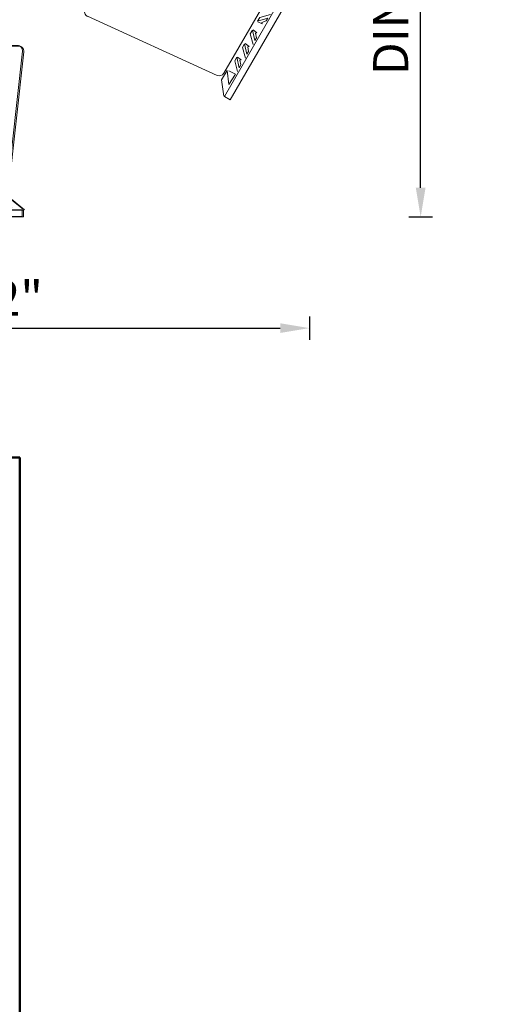
# Model space of a CAD drawing. Units: inches. Extents: x 1961 to 3038, y 800 to 1438.
# Tile 7 of 13: x 2803 to 2845, y 1012 to 1096. Entities that reach past the tile are written whole.
import ezdxf

# ---------------------------------------------------------------- set-up
doc = ezdxf.new("R2010")
doc.units = ezdxf.units.IN
for name, color, linetype, lineweight in [('A-ANNO-DIMS', 2, 'Continuous', 18), ('A-FURN', 8, 'Continuous', 18), ('A-WALL', 7, 'Continuous', 50)]:
    doc.layers.add(name, color=color, linetype=linetype, lineweight=lineweight)
doc.styles.get("Standard").update_dxf_attribs({"font": 'arial.ttf'})
doc.dimstyles.new('ISO-25', dxfattribs={"dimtxt": 3, "dimasz": 2.5, "dimexe": 1, "dimexo": 1, "dimtad": 1, "dimdec": 4, "dimlunit": 4, "dimtxsty": 'Standard', "dimcen": 2.5, "dimadec": 0, "dimazin": 0, "dimtfac": 1, "dimtdec": 4, "dimtmove": 0, "dimatfit": 3, "dimfxl": 1, "dimfxlon": 1, "dimarcsym": 0})

# ---------------------------------------------------------------- blocks, each defined once
blk = doc.blocks.new('A$C1C317F9A')
for p, q in [((0.8788, 2.2685), (0.8788, 2.2478)), ((1.3449, 2.2685), (0.8788, 2.2685)), ((1.3449, 2.2478), (1.3449, 2.2685)), ((0.8756, 2.2462), (0.9155, 2.2143)), ((0.8788, 2.2478), (1.3449, 2.2478)), ((0.9139, 2.2414), (0.9522, 2.243)), ((0.949, 2.2159), (0.9139, 2.2414)), ((0.9522, 2.243), (0.9506, 2.2206)), ((0.9618, 2.2446), (0.9857, 2.2206)), ((0.9745, 2.243), (0.9841, 2.243)), ((0.9985, 2.2206), (0.9745, 2.243)), ((0.9841, 2.243), (0.9953, 2.2334)), ((0.9953, 2.2334), (0.9985, 2.2366)), ((0.9985, 2.2366), (1.0001, 2.2222)), ((1.0097, 2.2446), (1.0336, 2.2206)), ((1.0224, 2.243), (1.032, 2.243)), ((1.0464, 2.2206), (1.0224, 2.243)), ((1.032, 2.243), (1.0432, 2.2334)), ((1.0432, 2.2334), (1.0464, 2.2366)), ((1.0464, 2.2366), (1.048, 2.2222)), ((1.0576, 2.2446), (1.0815, 2.2206)), ((1.0703, 2.243), (1.0799, 2.243)), ((1.0943, 2.2206), (1.0703, 2.243)), ((1.0799, 2.243), (1.0911, 2.2334)), ((1.0911, 2.2334), (1.0943, 2.2366)), ((1.0943, 2.2366), (1.0959, 2.2222)), ((1.1262, 2.2366), (1.1246, 2.2222)), ((1.1262, 2.2206), (1.1502, 2.243)), ((1.1294, 2.2334), (1.1262, 2.2366)), ((1.1406, 2.243), (1.1294, 2.2334)), ((1.1629, 2.2446), (1.139, 2.2206)), ((1.1502, 2.243), (1.1406, 2.243)), ((1.1741, 2.2366), (1.1725, 2.2222)), ((1.1741, 2.2206), (1.1981, 2.243)), ((1.1773, 2.2334), (1.1741, 2.2366)), ((1.1885, 2.243), (1.1773, 2.2334)), ((1.2108, 2.2446), (1.1869, 2.2206)), ((1.1981, 2.243), (1.1885, 2.243)), ((1.222, 2.2366), (1.2204, 2.2222)), ((1.222, 2.2206), (1.246, 2.243)), ((1.2252, 2.2334), (1.222, 2.2366)), ((1.2364, 2.243), (1.2252, 2.2334)), ((1.2587, 2.2446), (1.2348, 2.2206)), ((1.246, 2.243), (1.2364, 2.243)), ((1.2683, 2.243), (1.2699, 2.2206)), ((1.3066, 2.2414), (1.2683, 2.243)), ((1.2715, 2.2159), (1.3066, 2.2414)), ((1.3449, 2.2462), (1.305, 2.2143)), ((0.9155, 2.2143), (0.949, 2.2159)), ((0.941, 2.2111), (1.2841, 2.2111)), ((0.9857, 2.2206), (0.9985, 2.2206)), ((1.0336, 2.2206), (1.0464, 2.2206)), ((1.0815, 2.2206), (1.0943, 2.2206)), ((1.139, 2.2206), (1.1262, 2.2206)), ((1.1869, 2.2206), (1.1741, 2.2206)), ((1.2348, 2.2206), (1.222, 2.2206)), ((1.305, 2.2143), (1.2715, 2.2159)), ((0.8775, 1.7628), (0.9251, 2.1968)), ((1.3, 2.1966), (1.3417, 1.7626)), ((0.2422, 1.9115), (0.0091, 1.5078)), ((0.0271, 1.4974), (0.2602, 1.9011)), ((0.2602, 1.9011), (0.2422, 1.9115)), ((0.2615, 1.9003), (0.2692, 1.8498)), ((1.9514, 1.8873), (1.9438, 1.8368)), ((1.9724, 1.8957), (1.9544, 1.8854)), ((1.9544, 1.8854), (2.1875, 1.4816)), ((2.2055, 1.492), (1.9724, 1.8957)), ((0.2465, 1.8648), (0.226, 1.8324)), ((0.2511, 1.8216), (0.2465, 1.8648)), ((0.2692, 1.8498), (0.2511, 1.8216)), ((1.9619, 1.8086), (1.9665, 1.8518)), ((1.9665, 1.8518), (1.987, 1.8194)), ((0.09, 1.5329), (0.2615, 1.8301)), ((0.2148, 1.813), (0.21, 1.8047)), ((0.2222, 1.7811), (0.2148, 1.813)), ((0.2198, 1.8249), (0.2286, 1.7922)), ((0.226, 1.8324), (0.2461, 1.8226)), ((0.282, 1.8367), (0.6787, 1.6557)), ((1.5338, 1.644), (1.9335, 1.8198)), ((1.9438, 1.8368), (1.9619, 1.8086)), ((1.9537, 1.8131), (2.1253, 1.516)), ((1.987, 1.8194), (1.9669, 1.8096)), ((1.9932, 1.8119), (1.9844, 1.7792)), ((0.1959, 1.7834), (0.2046, 1.7507)), ((0.2127, 1.7903), (0.2084, 1.7891)), ((0.2084, 1.7891), (0.22, 1.7805)), ((0.21, 1.8047), (0.2127, 1.7903)), ((0.2286, 1.7922), (0.2222, 1.7811)), ((1.9844, 1.7792), (1.9908, 1.7681)), ((1.9908, 1.7681), (1.9982, 1.8)), ((1.9982, 1.8), (2.003, 1.7917)), ((2.003, 1.7917), (2.0003, 1.7773)), ((0.1888, 1.7488), (0.1844, 1.7476)), ((0.1909, 1.7716), (0.1861, 1.7633)), ((0.1861, 1.7633), (0.1888, 1.7488)), ((0.1982, 1.7396), (0.1909, 1.7716)), ((0.2046, 1.7507), (0.1982, 1.7396)), ((2.0046, 1.7761), (1.993, 1.7675)), ((2.0003, 1.7773), (2.0046, 1.7761)), ((2.0171, 1.7704), (2.0084, 1.7377)), ((2.0147, 1.7266), (2.0221, 1.7585)), ((2.0221, 1.7585), (2.0269, 1.7502)), ((2.0269, 1.7502), (2.0242, 1.7358)), ((0.1669, 1.7301), (0.1621, 1.7218)), ((0.1621, 1.7218), (0.1648, 1.7073)), ((0.1743, 1.6982), (0.1669, 1.7301)), ((0.1719, 1.7419), (0.1807, 1.7092)), ((0.1844, 1.7476), (0.1961, 1.7391)), ((1.3258, 1.7451), (0.8934, 1.7451)), ((2.0084, 1.7377), (2.0147, 1.7266)), ((2.0286, 1.7346), (2.0169, 1.726)), ((2.0242, 1.7358), (2.0286, 1.7346)), ((2.0411, 1.7289), (2.0323, 1.6962)), ((0.1648, 1.7073), (0.1605, 1.7061)), ((0.1605, 1.7061), (0.1721, 1.6976)), ((0.1807, 1.7092), (0.1743, 1.6982)), ((2.0323, 1.6962), (2.0387, 1.6852)), ((2.0387, 1.6852), (2.0461, 1.7171)), ((2.0525, 1.6931), (2.0409, 1.6846)), ((2.0461, 1.7171), (2.0509, 1.7088)), ((2.0509, 1.7088), (2.0482, 1.6943)), ((2.0482, 1.6943), (2.0525, 1.6931)), ((0.1192, 1.6507), (0.1519, 1.6595)), ((0.1583, 1.6705), (0.127, 1.6609)), ((0.127, 1.6609), (0.1318, 1.6692)), ((0.1318, 1.6692), (0.1457, 1.6741)), ((0.1445, 1.6785), (0.1577, 1.6727)), ((0.1457, 1.6741), (0.1445, 1.6785)), ((0.1519, 1.6595), (0.1583, 1.6705)), ((2.0685, 1.6655), (2.0552, 1.6597)), ((2.0673, 1.6611), (2.0685, 1.6655)), ((2.0812, 1.6562), (2.0673, 1.6611)), ((0.1344, 1.629), (0.1031, 1.6195)), ((0.1078, 1.6278), (0.1217, 1.6327)), ((0.1217, 1.6327), (0.1206, 1.637)), ((0.1206, 1.637), (0.1338, 1.6312)), ((0.128, 1.618), (0.1344, 1.629)), ((0.6859, 1.6332), (0.4697, 1.2588)), ((1.091, 1.6437, 0.0908), (1.091, 1.4528, 0.0908)), ((1.097, 1.6437, 0.0908), (1.091, 1.6437, 0.0908)), ((1.097, 1.4528, 0.0908), (1.097, 1.6437, 0.0908)), ((1.1023, 1.6437, 0.0908), (1.1023, 1.4528, 0.0908)), ((1.1083, 1.6437, 0.0908), (1.1023, 1.6437, 0.0908)), ((1.1083, 1.4528, 0.0908), (1.1083, 1.6437, 0.0908)), ((2.0547, 1.6575), (2.086, 1.6479)), ((2.061, 1.6464), (2.0547, 1.6575)), ((2.0937, 1.6377), (2.061, 1.6464)), ((2.086, 1.6479), (2.0812, 1.6562)), ((0.0953, 1.6092), (0.128, 1.618)), ((0.1031, 1.6195), (0.1078, 1.6278)), ((1.7426, 1.2469), (1.5264, 1.6214)), ((2.0786, 1.616), (2.1099, 1.6065)), ((2.085, 1.605), (2.0786, 1.616)), ((2.0924, 1.624), (2.0792, 1.6182)), ((2.1177, 1.5962), (2.085, 1.605)), ((2.0913, 1.6196), (2.0924, 1.624)), ((2.1051, 1.6148), (2.0913, 1.6196)), ((2.1099, 1.6065), (2.1051, 1.6148)), ((0.0713, 1.5677), (0.104, 1.5765)), ((0.1104, 1.5876), (0.0791, 1.578)), ((0.0791, 1.578), (0.0839, 1.5863)), ((0.0839, 1.5863), (0.0978, 1.5912)), ((0.0966, 1.5955), (0.1098, 1.5897)), ((0.0978, 1.5912), (0.0966, 1.5955)), ((0.104, 1.5765), (0.1104, 1.5876)), ((2.1026, 1.5745), (2.1339, 1.565)), ((2.1089, 1.5635), (2.1026, 1.5745)), ((2.1164, 1.5825), (2.1031, 1.5767)), ((2.1152, 1.5782), (2.1164, 1.5825)), ((2.1291, 1.5733), (2.1152, 1.5782)), ((2.1339, 1.565), (2.1291, 1.5733)), ((0.0502, 1.5246), (0.0679, 1.5586)), ((0.0898, 1.5423), (0.0502, 1.5246)), ((0.0679, 1.5586), (0.0865, 1.5461)), ((0.0745, 1.5125), (0.0898, 1.5423)), ((2.1416, 1.5547), (2.1089, 1.5635)), ((2.145, 1.5456), (2.1265, 1.5331)), ((2.1628, 1.5116), (2.145, 1.5456)), ((0.0091, 1.5078), (0.0271, 1.4974)), ((0.0269, 1.4939), (0.0745, 1.5125)), ((0.4464, 1.2539), (0.0943, 1.5121)), ((2.1232, 1.5293), (2.1628, 1.5116)), ((2.1385, 1.4995), (2.1232, 1.5293)), ((1.0755, 1.4796, 0.0908), (1.0755, 1.4641, 0.0908)), ((1.091, 1.4796, 0.0908), (1.0755, 1.4796, 0.0908)), ((1.1023, 1.4796, 0.0908), (1.097, 1.4796, 0.0908)), ((1.125, 1.4796, 0.0908), (1.1083, 1.4796, 0.0908)), ((1.125, 1.4641, 0.0908), (1.125, 1.4796, 0.0908)), ((2.1208, 1.495), (1.7657, 1.2419)), ((2.1861, 1.4809), (2.1385, 1.4995)), ((2.1875, 1.4816), (2.2055, 1.492)), ((1.0755, 1.4641, 0.0908), (1.091, 1.4641, 0.0908)), ((1.091, 1.4528, 0.0908), (1.097, 1.4528, 0.0908)), ((1.097, 1.4641, 0.0908), (1.1023, 1.4641, 0.0908)), ((1.1023, 1.4528, 0.0908), (1.1083, 1.4528, 0.0908)), ((1.1083, 1.4641, 0.0908), (1.125, 1.4641, 0.0908)), ((0.9684, 1.4231, 0.0908), (0.9184, 1.3706, 0.0908)), ((0.953, 1.3489, 0.0908), (0.9684, 1.4231, 0.0908)), ((1.1549, 1.429, 0.0908), (1.0933, 1.4112, 0.0908)), ((1.1882, 1.4134, 0.0908), (1.1549, 1.429, 0.0908)), ((1.2075, 1.4282, 0.0908), (1.1882, 1.4134, 0.0908)), ((1.278, 1.4112, 0.0908), (1.2075, 1.4282, 0.0908)), ((0.6822, 1.3924, 0.0908), (0.6792, 1.3872, 0.0908)), ((0.6792, 1.3872, 0.0908), (0.8446, 1.2917, 0.0908)), ((0.8476, 1.2969, 0.0908), (0.6822, 1.3924, 0.0908)), ((1.0933, 1.4112, 0.0908), (1.1623, 1.3815, 0.0908)), ((1.1623, 1.3815, 0.0908), (1.2061, 1.3874, 0.0908)), ((1.2061, 1.3874, 0.0908), (1.278, 1.4112, 0.0908)), ((1.5304, 1.4154, 0.0908), (1.365, 1.3199, 0.0908)), ((1.368, 1.3147, 0.0908), (1.5334, 1.4102, 0.0908)), ((1.5361, 1.4055, 0.0908), (1.3707, 1.3101, 0.0908)), ((1.3737, 1.3049, 0.0908), (1.539, 1.4004, 0.0908)), ((1.5334, 1.4102, 0.0908), (1.5304, 1.4154, 0.0908)), ((1.539, 1.4004, 0.0908), (1.5361, 1.4055, 0.0908)), ((0.6765, 1.3825, 0.0908), (0.6735, 1.3774, 0.0908)), ((0.6735, 1.3774, 0.0908), (0.8389, 1.2819, 0.0908)), ((0.8419, 1.2871, 0.0908), (0.6765, 1.3825, 0.0908)), ((0.9184, 1.3706, 0.0908), (0.9216, 1.3464, 0.0908)), ((0.9216, 1.3464, 0.0908), (0.8914, 1.3253, 0.0908)), ((0.9363, 1.308, 0.0908), (0.953, 1.3489, 0.0908)), ((1.3805, 1.3467, 0.0908), (1.3671, 1.339, 0.0908)), ((1.3671, 1.339, 0.0908), (1.3748, 1.3255, 0.0908)), ((1.3883, 1.3333, 0.0908), (1.3805, 1.3467, 0.0908)), ((1.3939, 1.3235, 0.0908), (1.3912, 1.3281, 0.0908)), ((0.8213, 1.3051, 0.0908), (0.8186, 1.3005, 0.0908)), ((0.8327, 1.3248, 0.0908), (0.8243, 1.3103, 0.0908)), ((0.8321, 1.2927, 0.0908), (0.8348, 1.2974, 0.0908)), ((0.8461, 1.317, 0.0908), (0.8327, 1.3248, 0.0908)), ((0.8377, 1.3025, 0.0908), (0.8461, 1.317, 0.0908)), ((0.8446, 1.2917, 0.0908), (0.8476, 1.2969, 0.0908)), ((0.8914, 1.3253, 0.0908), (0.8761, 1.2631, 0.0908)), ((0.8761, 1.2631, 0.0908), (0.9363, 1.308, 0.0908)), ((1.3763, 1.2527, 0.0908), (1.3301, 1.2971, 0.0908)), ((1.3301, 1.2971, 0.0908), (1.3389, 1.2225, 0.0908)), ((1.365, 1.3199, 0.0908), (1.368, 1.3147, 0.0908)), ((1.3707, 1.3101, 0.0908), (1.3737, 1.3049, 0.0908)), ((1.3778, 1.3204, 0.0908), (1.3805, 1.3157, 0.0908)), ((1.3835, 1.3106, 0.0908), (1.3918, 1.2961, 0.0908)), ((1.3918, 1.2961, 0.0908), (1.4053, 1.3038, 0.0908)), ((1.4053, 1.3038, 0.0908), (1.3969, 1.3183, 0.0908)), ((0.8156, 1.2953, 0.0908), (0.8079, 1.2819, 0.0908)), ((0.8079, 1.2819, 0.0908), (0.8213, 1.2741, 0.0908)), ((0.8213, 1.2741, 0.0908), (0.8291, 1.2876, 0.0908)), ((0.8389, 1.2819, 0.0908), (0.8419, 1.2871, 0.0908)), ((1.3795, 1.216, 0.0908), (1.3763, 1.2527, 0.0908)), ((1.3389, 1.2225, 0.0908), (1.366, 1.1876, 0.0908)), ((1.402, 1.2067, 0.0908), (1.3795, 1.216, 0.0908)), ((1.4225, 1.1371, 0.0908), (1.402, 1.2067, 0.0908)), ((1.366, 1.1876, 0.0908), (1.4225, 1.1371, 0.0908)), ((0.8033, 1.1609, 0.0908), (0.8238, 1.0913, 0.0908)), ((0.8599, 1.1105, 0.0908), (0.8033, 1.1609, 0.0908)), ((0.8238, 1.0913, 0.0908), (0.8463, 1.0821, 0.0908)), ((0.8869, 1.0755, 0.0908), (0.8599, 1.1105, 0.0908)), ((0.8463, 1.0821, 0.0908), (0.8495, 1.0454, 0.0908)), ((0.8957, 1.0009, 0.0908), (0.8869, 1.0755, 0.0908)), ((0.0847, 0.7751), (0.4398, 1.0281)), ((0.8495, 1.0454, 0.0908), (0.8957, 1.0009, 0.0908)), ((1.3498, 1.0349, 0.0908), (1.2896, 0.99, 0.0908)), ((1.3344, 0.9727, 0.0908), (1.3498, 1.0349, 0.0908)), ((0.4628, 1.0231), (0.679, 0.6486)), ((0.834, 1.0019, 0.0908), (0.8206, 0.9942, 0.0908)), ((0.8424, 0.9875, 0.0908), (0.834, 1.0019, 0.0908)), ((1.3813, 1.0063, 0.0908), (1.3783, 1.0011, 0.0908)), ((1.3783, 1.0011, 0.0908), (1.5437, 0.9057, 0.0908)), ((1.3881, 0.9955, 0.0908), (1.3797, 0.981, 0.0908)), ((1.5466, 0.9108, 0.0908), (1.3813, 1.0063, 0.0908)), ((1.3869, 1.0161, 0.0908), (1.384, 1.011, 0.0908)), ((1.384, 1.011, 0.0908), (1.5493, 0.9155, 0.0908)), ((1.5523, 0.9207, 0.0908), (1.3869, 1.0161, 0.0908)), ((1.3938, 1.0053, 0.0908), (1.3911, 1.0006, 0.0908)), ((1.4045, 1.0239, 0.0908), (1.3968, 1.0105, 0.0908)), ((1.418, 1.0162, 0.0908), (1.4045, 1.0239, 0.0908)), ((1.4045, 0.9929, 0.0908), (1.4072, 0.9975, 0.0908)), ((1.4102, 1.0027, 0.0908), (1.418, 1.0162, 0.0908)), ((1.5196, 0.6368), (1.7358, 1.0113)), ((1.7591, 1.0162), (2.1111, 0.7579)), ((0.8522, 0.9931, 0.0908), (0.6868, 0.8977, 0.0908)), ((0.6898, 0.8925, 0.0908), (0.8552, 0.988, 0.0908)), ((0.8578, 0.9833, 0.0908), (0.6925, 0.8878, 0.0908)), ((0.6955, 0.8827, 0.0908), (0.8608, 0.9781, 0.0908)), ((0.8206, 0.9942, 0.0908), (0.8289, 0.9797, 0.0908)), ((0.8319, 0.9745, 0.0908), (0.8346, 0.9699, 0.0908)), ((0.8376, 0.9647, 0.0908), (0.8453, 0.9513, 0.0908)), ((0.848, 0.9776, 0.0908), (0.8453, 0.9823, 0.0908)), ((0.8588, 0.959, 0.0908), (0.851, 0.9725, 0.0908)), ((0.8552, 0.988, 0.0908), (0.8522, 0.9931, 0.0908)), ((0.8608, 0.9781, 0.0908), (0.8578, 0.9833, 0.0908)), ((1.2896, 0.99, 0.0908), (1.2728, 0.9491, 0.0908)), ((1.3042, 0.9516, 0.0908), (1.3344, 0.9727, 0.0908)), ((1.3797, 0.981, 0.0908), (1.3932, 0.9732, 0.0908)), ((1.3932, 0.9732, 0.0908), (1.4015, 0.9877, 0.0908)), ((0.8453, 0.9513, 0.0908), (0.8588, 0.959, 0.0908)), ((1.2728, 0.9491, 0.0908), (1.2574, 0.875, 0.0908)), ((1.3074, 0.9275, 0.0908), (1.3042, 0.9516, 0.0908)), ((1.0198, 0.9106, 0.0908), (0.9478, 0.8869, 0.0908)), ((1.0636, 0.9165, 0.0908), (1.0198, 0.9106, 0.0908)), ((1.1326, 0.8869, 0.0908), (1.0636, 0.9165, 0.0908)), ((1.2574, 0.875, 0.0908), (1.3074, 0.9275, 0.0908)), ((1.5437, 0.9057, 0.0908), (1.5466, 0.9108, 0.0908)), ((1.5493, 0.9155, 0.0908), (1.5523, 0.9207, 0.0908)), ((0.6868, 0.8977, 0.0908), (0.6898, 0.8925, 0.0908)), ((0.6925, 0.8878, 0.0908), (0.6955, 0.8827, 0.0908)), ((0.9478, 0.8869, 0.0908), (1.0183, 0.8698, 0.0908)), ((1.0183, 0.8698, 0.0908), (1.0376, 0.8846, 0.0908)), ((1.0376, 0.8846, 0.0908), (1.071, 0.8691, 0.0908)), ((1.071, 0.8691, 0.0908), (1.1326, 0.8869, 0.0908)), ((1.1235, 0.8453, 0.0908), (1.1175, 0.8453, 0.0908)), ((1.1175, 0.8453, 0.0908), (1.1175, 0.6543, 0.0908)), ((1.1235, 0.6543, 0.0908), (1.1235, 0.8453, 0.0908)), ((1.1349, 0.8453, 0.0908), (1.1289, 0.8453, 0.0908)), ((1.1289, 0.8453, 0.0908), (1.1289, 0.6543, 0.0908)), ((1.1349, 0.6543, 0.0908), (1.1349, 0.8453, 0.0908)), ((1.1175, 0.8339, 0.0908), (1.1008, 0.8339, 0.0908)), ((1.1008, 0.8339, 0.0908), (1.1008, 0.8184, 0.0908)), ((1.1008, 0.8184, 0.0908), (1.1175, 0.8184, 0.0908)), ((1.1289, 0.8339, 0.0908), (1.1235, 0.8339, 0.0908)), ((1.1235, 0.8184, 0.0908), (1.1289, 0.8184, 0.0908)), ((1.1504, 0.8339, 0.0908), (1.1349, 0.8339, 0.0908)), ((1.1349, 0.8184, 0.0908), (1.1504, 0.8184, 0.0908)), ((1.1504, 0.8184, 0.0908), (1.1504, 0.8339, 0.0908)), ((0.018, 0.7884), (0, 0.778)), ((0.2511, 0.3847), (0.018, 0.7884)), ((0.0193, 0.7892), (0.0669, 0.7706)), ((0, 0.778), (0.2331, 0.3743)), ((0.0427, 0.7584), (0.0604, 0.7244)), ((0.0823, 0.7407), (0.0427, 0.7584)), ((0.0669, 0.7706), (0.0823, 0.7407)), ((0.2517, 0.4569), (0.0802, 0.7541)), ((2.1784, 0.7726), (1.9453, 0.3689)), ((1.9633, 0.3585), (2.1964, 0.7622)), ((2.131, 0.7576), (2.1156, 0.7277)), ((2.1786, 0.7762), (2.131, 0.7576)), ((2.1964, 0.7622), (2.1784, 0.7726)), ((0.0604, 0.7244), (0.079, 0.737)), ((2.1155, 0.7371), (1.9439, 0.4399)), ((2.1156, 0.7277), (2.1553, 0.7454)), ((2.1375, 0.7114), (2.119, 0.724)), ((2.1553, 0.7454), (2.1375, 0.7114)), ((0.0638, 0.7153), (0.0965, 0.7066)), ((0.0716, 0.7051), (0.0764, 0.6968)), ((0.1029, 0.6955), (0.0716, 0.7051)), ((0.0764, 0.6968), (0.0903, 0.6919)), ((0.0965, 0.7066), (0.1029, 0.6955)), ((2.1014, 0.6935), (2.095, 0.6825)), ((2.1341, 0.7023), (2.1014, 0.6935)), ((0.0878, 0.6738), (0.1205, 0.6651)), ((0.0891, 0.6875), (0.1023, 0.6933)), ((0.0903, 0.6919), (0.0891, 0.6875)), ((0.0955, 0.6636), (0.1003, 0.6553)), ((0.1269, 0.654), (0.0955, 0.6636)), ((0.1205, 0.6651), (0.1269, 0.654)), ((2.095, 0.6825), (2.1264, 0.6921)), ((2.1089, 0.6745), (2.0956, 0.6803)), ((2.1216, 0.6838), (2.1077, 0.6789)), ((2.1077, 0.6789), (2.1089, 0.6745)), ((2.1264, 0.6921), (2.1216, 0.6838)), ((0.1003, 0.6553), (0.1142, 0.6504)), ((0.1131, 0.646), (0.1263, 0.6518)), ((0.1142, 0.6504), (0.1131, 0.646)), ((1.1175, 0.6543, 0.0908), (1.1235, 0.6543, 0.0908)), ((1.1289, 0.6543, 0.0908), (1.1349, 0.6543, 0.0908)), ((2.0775, 0.6521), (2.0711, 0.641)), ((2.0711, 0.641), (2.1024, 0.6506)), ((2.0849, 0.633), (2.0717, 0.6388)), ((2.1102, 0.6608), (2.0775, 0.6521)), ((2.0976, 0.6423), (2.0837, 0.6374)), ((2.0837, 0.6374), (2.0849, 0.633)), ((2.1024, 0.6506), (2.0976, 0.6423)), ((0.1117, 0.6324), (0.1444, 0.6236)), ((0.1195, 0.6221), (0.1243, 0.6138)), ((0.1508, 0.6125), (0.1195, 0.6221)), ((0.1243, 0.6138), (0.1382, 0.6089)), ((0.137, 0.6046), (0.1502, 0.6104)), ((0.1382, 0.6089), (0.137, 0.6046)), ((0.1444, 0.6236), (0.1508, 0.6125)), ((0.6716, 0.6261), (0.272, 0.4503)), ((1.9235, 0.4334), (1.5268, 0.6143)), ((2.0535, 0.6106), (2.0471, 0.5995)), ((2.0471, 0.5995), (2.0785, 0.6091)), ((2.0862, 0.6194), (2.0535, 0.6106)), ((2.0785, 0.6091), (2.0737, 0.6008)), ((0.153, 0.5769), (0.1646, 0.5855)), ((0.1573, 0.5757), (0.153, 0.5769)), ((0.1546, 0.5613), (0.1573, 0.5757)), ((0.1668, 0.5849), (0.1594, 0.553)), ((0.1644, 0.5411), (0.1732, 0.5738)), ((0.1732, 0.5738), (0.1668, 0.5849)), ((2.061, 0.5915), (2.0477, 0.5973)), ((2.0737, 0.6008), (2.0598, 0.5959)), ((2.0598, 0.5959), (2.061, 0.5915)), ((0.1594, 0.553), (0.1546, 0.5613)), ((0.1769, 0.5354), (0.1885, 0.544)), ((0.1907, 0.5434), (0.1834, 0.5115)), ((0.1971, 0.5323), (0.1907, 0.5434)), ((2.0248, 0.5608), (2.0312, 0.5719)), ((2.0336, 0.5281), (2.0248, 0.5608)), ((2.0312, 0.5719), (2.0386, 0.54)), ((2.045, 0.5639), (2.0334, 0.5725)), ((2.0386, 0.54), (2.0433, 0.5483)), ((2.0406, 0.5627), (2.045, 0.5639)), ((2.0433, 0.5483), (2.0406, 0.5627)), ((0.1813, 0.5343), (0.1769, 0.5354)), ((0.1786, 0.5198), (0.1813, 0.5343)), ((0.1834, 0.5115), (0.1786, 0.5198)), ((0.1884, 0.4996), (0.1971, 0.5323)), ((0.8797, 0.5249), (1.3121, 0.5249)), ((0.8838, 0.5234), (1.3162, 0.5234)), ((2.0009, 0.5193), (2.0072, 0.5304)), ((2.0096, 0.4866), (2.0009, 0.5193)), ((2.0072, 0.5304), (2.0146, 0.4985)), ((2.0211, 0.5224), (2.0094, 0.531)), ((2.0167, 0.5212), (2.0211, 0.5224)), ((2.0194, 0.5068), (2.0167, 0.5212)), ((0.2009, 0.4939), (0.2125, 0.5025)), ((0.2052, 0.4928), (0.2009, 0.4939)), ((0.2025, 0.4783), (0.2052, 0.4928)), ((0.2147, 0.5019), (0.2073, 0.47)), ((0.2123, 0.4582), (0.2211, 0.4909)), ((0.2211, 0.4909), (0.2147, 0.5019)), ((0.9055, 0.0734), (0.8638, 0.5074)), ((0.9096, 0.0719), (0.8679, 0.5059)), ((1.328, 0.5072), (1.2804, 0.0732)), ((1.3321, 0.5057), (1.2845, 0.0717)), ((1.9769, 0.4779), (1.9833, 0.4889)), ((1.9833, 0.4889), (1.9907, 0.457)), ((1.9971, 0.4809), (1.9855, 0.4895)), ((2.0146, 0.4985), (2.0194, 0.5068)), ((0.2073, 0.47), (0.2025, 0.4783)), ((0.2185, 0.4507), (0.2386, 0.4604)), ((0.2436, 0.4615), (0.239, 0.4183)), ((0.2617, 0.4332), (0.2436, 0.4615)), ((1.9857, 0.4451), (1.9769, 0.4779)), ((1.9907, 0.457), (1.9955, 0.4653)), ((1.9927, 0.4798), (1.9971, 0.4809)), ((1.9955, 0.4653), (1.9927, 0.4798)), ((0.239, 0.4183), (0.2185, 0.4507)), ((0.254, 0.3827), (0.2617, 0.4332)), ((1.9363, 0.4202), (1.9544, 0.4484)), ((1.9544, 0.4484), (1.9589, 0.4053)), ((1.9589, 0.4053), (1.9795, 0.4377)), ((1.9795, 0.4377), (1.9593, 0.4474)), ((1.9439, 0.3697), (1.9363, 0.4202)), ((0.2331, 0.3743), (0.2511, 0.3847)), ((1.9453, 0.3689), (1.9633, 0.3585)), ((0.8605, 0.0239), (0.9005, 0.0558)), ((0.8647, 0.0223), (0.9046, 0.0543)), ((0.934, 0.0542), (0.8989, 0.0286)), ((0.9005, 0.0558), (0.934, 0.0542)), ((0.9381, 0.0527), (0.903, 0.0271)), ((0.9046, 0.0543), (0.9381, 0.0527)), ((1.2645, 0.059), (0.9213, 0.059)), ((1.2686, 0.0574), (0.9255, 0.0574)), ((0.9372, 0.027), (0.9356, 0.0494)), ((0.9413, 0.0255), (0.9397, 0.0479)), ((0.9468, 0.0255), (0.9707, 0.0494)), ((0.9509, 0.0239), (0.9748, 0.0479)), ((0.9835, 0.0494), (0.9595, 0.027)), ((0.9876, 0.0479), (0.9636, 0.0255)), ((0.9691, 0.027), (0.9803, 0.0366)), ((0.9707, 0.0494), (0.9835, 0.0494)), ((0.9732, 0.0255), (0.9844, 0.0351)), ((0.9748, 0.0479), (0.9876, 0.0479)), ((0.9803, 0.0366), (0.9835, 0.0334)), ((0.9835, 0.0334), (0.9851, 0.0478)), ((0.9844, 0.0351), (0.9876, 0.0319)), ((0.9876, 0.0319), (0.9892, 0.0463)), ((0.9946, 0.0255), (1.0186, 0.0494)), ((0.9988, 0.0239), (1.0227, 0.0479)), ((1.0314, 0.0494), (1.0074, 0.027)), ((1.0355, 0.0479), (1.0115, 0.0255)), ((1.017, 0.027), (1.0282, 0.0366)), ((1.0186, 0.0494), (1.0314, 0.0494)), ((1.0211, 0.0255), (1.0323, 0.0351)), ((1.0227, 0.0479), (1.0355, 0.0479)), ((1.0282, 0.0366), (1.0314, 0.0334)), ((1.0314, 0.0334), (1.033, 0.0478)), ((1.0323, 0.0351), (1.0355, 0.0319)), ((1.0355, 0.0319), (1.0371, 0.0463)), ((1.0425, 0.0255), (1.0665, 0.0494)), ((1.0467, 0.0239), (1.0706, 0.0479)), ((1.0793, 0.0494), (1.0553, 0.027)), ((1.0834, 0.0479), (1.0594, 0.0255)), ((1.0649, 0.027), (1.0761, 0.0366)), ((1.0665, 0.0494), (1.0793, 0.0494)), ((1.069, 0.0255), (1.0802, 0.0351)), ((1.0706, 0.0479), (1.0834, 0.0479)), ((1.0761, 0.0366), (1.0793, 0.0334)), ((1.0793, 0.0334), (1.0809, 0.0478)), ((1.0802, 0.0351), (1.0834, 0.0319)), ((1.0834, 0.0319), (1.085, 0.0463)), ((1.1112, 0.0334), (1.1096, 0.0478)), ((1.1112, 0.0494), (1.1351, 0.027)), ((1.124, 0.0494), (1.1112, 0.0494)), ((1.1144, 0.0366), (1.1112, 0.0334)), ((1.1153, 0.0319), (1.1137, 0.0463)), ((1.1256, 0.027), (1.1144, 0.0366)), ((1.1153, 0.0479), (1.1393, 0.0255)), ((1.1281, 0.0479), (1.1153, 0.0479)), ((1.1185, 0.0351), (1.1153, 0.0319)), ((1.1297, 0.0255), (1.1185, 0.0351)), ((1.1479, 0.0255), (1.124, 0.0494)), ((1.152, 0.0239), (1.1281, 0.0479)), ((1.1591, 0.0334), (1.1575, 0.0478)), ((1.1591, 0.0494), (1.183, 0.027)), ((1.1719, 0.0494), (1.1591, 0.0494)), ((1.1623, 0.0366), (1.1591, 0.0334)), ((1.1632, 0.0319), (1.1616, 0.0463)), ((1.1735, 0.027), (1.1623, 0.0366)), ((1.1632, 0.0479), (1.1872, 0.0255)), ((1.176, 0.0479), (1.1632, 0.0479)), ((1.1664, 0.0351), (1.1632, 0.0319)), ((1.1776, 0.0255), (1.1664, 0.0351)), ((1.1958, 0.0255), (1.1719, 0.0494)), ((1.1999, 0.0239), (1.176, 0.0479)), ((1.207, 0.0334), (1.2054, 0.0478)), ((1.207, 0.0494), (1.2309, 0.027)), ((1.2198, 0.0494), (1.207, 0.0494)), ((1.2102, 0.0366), (1.207, 0.0334)), ((1.2111, 0.0319), (1.2095, 0.0463)), ((1.2214, 0.027), (1.2102, 0.0366)), ((1.2111, 0.0479), (1.235, 0.0255)), ((1.2239, 0.0479), (1.2111, 0.0479)), ((1.2143, 0.0351), (1.2111, 0.0319)), ((1.2255, 0.0255), (1.2143, 0.0351)), ((1.2437, 0.0255), (1.2198, 0.0494)), ((1.2478, 0.0239), (1.2239, 0.0479)), ((1.2533, 0.027), (1.2549, 0.0494)), ((1.29, 0.0558), (1.2565, 0.0542)), ((1.2565, 0.0542), (1.2916, 0.0286)), ((1.2574, 0.0255), (1.259, 0.0479)), ((1.2941, 0.0543), (1.2606, 0.0527)), ((1.2606, 0.0527), (1.2957, 0.0271)), ((1.3299, 0.0239), (1.29, 0.0558)), ((1.334, 0.0223), (1.2941, 0.0543)), ((0.8605, 0.0223), (0.8605, 0.0015)), ((1.3267, 0.0223), (0.8605, 0.0223)), ((0.8605, 0.0015), (1.3267, 0.0015)), ((0.8647, 0.0207), (0.8647, 0)), ((1.3308, 0.0207), (0.8647, 0.0207)), ((0.8647, 0), (1.3308, 0)), ((0.8989, 0.0286), (0.9372, 0.027)), ((0.903, 0.0271), (0.9413, 0.0255)), ((0.9595, 0.027), (0.9691, 0.027)), ((0.9636, 0.0255), (0.9732, 0.0255)), ((1.0074, 0.027), (1.017, 0.027)), ((1.0115, 0.0255), (1.0211, 0.0255)), ((1.0553, 0.027), (1.0649, 0.027)), ((1.0594, 0.0255), (1.069, 0.0255)), ((1.1351, 0.027), (1.1256, 0.027)), ((1.1393, 0.0255), (1.1297, 0.0255)), ((1.183, 0.027), (1.1735, 0.027)), ((1.1872, 0.0255), (1.1776, 0.0255)), ((1.2309, 0.027), (1.2214, 0.027)), ((1.235, 0.0255), (1.2255, 0.0255)), ((1.2916, 0.0286), (1.2533, 0.027)), ((1.2957, 0.0271), (1.2574, 0.0255)), ((1.3267, 0.0015), (1.3267, 0.0223)), ((1.3308, 0), (1.3308, 0.0207))]:
    blk.add_line(p, q)
for centre, radius in [((1.1027, 1.135), 0.537), ((1.1027, 1.135), 0.527), ((1.0059, 1.525, 0.0908), 0.0569), ((1.1975, 1.5297, 0.0908), 0.0613), ((1.0072, 1.5257, 0.0908), 0.0294), ((1.385, 1.4297, 0.0908), 0.0569), ((0.8256, 1.4126, 0.0908), 0.0613), ((1.3863, 1.4289, 0.0908), 0.0294), ((1.4849, 1.2661, 0.0908), 0.0613), ((0.7338, 1.2443, 0.0908), 0.0569), ((0.7339, 1.2458, 0.0908), 0.0294), ((0.741, 1.0319, 0.0908), 0.0613), ((1.4921, 1.0537, 0.0908), 0.0569), ((1.492, 1.0522, 0.0908), 0.0294), ((1.4003, 0.8854, 0.0908), 0.0613), ((0.8408, 0.8683, 0.0908), 0.0569), ((0.8396, 0.8691, 0.0908), 0.0294), ((1.0283, 0.7683, 0.0908), 0.0613), ((1.2199, 0.773, 0.0908), 0.0569), ((1.2186, 0.7723, 0.0908), 0.0294)]:
    blk.add_circle(centre, radius)
for centre, radius, start, end in [((0.941, 2.1951), 0.016, 90, 173.7428), ((1.2841, 2.1951), 0.016, 5.4801, 90), ((0.2754, 1.8222), 0.016, 65.4801, 150), ((1.9399, 1.8052), 0.016, 30, 113.7428), ((0.8934, 1.7611), 0.016, 173.7428, 270), ((1.3258, 1.7611), 0.016, 270, 5.4801), ((0.6721, 1.6412), 0.016, 330, 65.4801), ((1.5403, 1.6294), 0.016, 113.7428, 210), ((0.1038, 1.525), 0.016, 150, 233.7428), ((2.1115, 1.508), 0.016, 305.4801, 30), ((1.1801, 1.4052, 0.0908), 0.0446, 26.6641, 154.1442), ((1.1801, 1.4052, 0.0908), 0.0446, 197.0611, 344.0662), ((0.9246, 1.3353, 0.0908), 0.0446, 86.6641, 214.1442), ((0.9246, 1.3353, 0.0908), 0.0446, 257.0611, 44.0662), ((0.4559, 1.2667), 0.016, 233.7428, 330), ((1.3684, 1.2189, 0.0908), 0.0446, 137.0611, 284.0662), ((1.3684, 1.2189, 0.0908), 0.0446, 326.6641, 94.1442), ((1.7565, 1.2549), 0.016, 210, 305.4801), ((0.8574, 1.0791, 0.0908), 0.0446, 317.0611, 104.0662), ((0.8574, 1.0791, 0.0908), 0.0446, 146.6641, 274.1442), ((0.449, 1.0151), 0.016, 30, 125.4801), ((1.3012, 0.9627, 0.0908), 0.0446, 77.0611, 224.0662), ((1.7496, 1.0033), 0.016, 53.7428, 150), ((1.3012, 0.9627, 0.0908), 0.0446, 266.6641, 34.1442), ((1.0457, 0.8928, 0.0908), 0.0446, 17.0611, 164.0662), ((1.0457, 0.8928, 0.0908), 0.0446, 206.6641, 334.1442), ((0.094, 0.7621), 0.016, 125.4801, 210), ((2.1017, 0.7451), 0.016, 330, 53.7428), ((0.6652, 0.6407), 0.016, 293.7428, 30), ((1.5334, 0.6288), 0.016, 150, 245.4801), ((0.8797, 0.5089), 0.016, 90, 185.4801), ((0.8838, 0.5074), 0.016, 90, 185.4801), ((1.3121, 0.5089), 0.016, 353.7428, 90), ((1.3162, 0.5074), 0.016, 353.7428, 90), ((0.2656, 0.4649), 0.016, 210, 293.7428), ((1.9301, 0.4479), 0.016, 245.4801, 330), ((0.9213, 0.0749), 0.016, 185.4801, 270), ((0.9255, 0.0734), 0.016, 185.4801, 270), ((1.2645, 0.0749), 0.016, 270, 353.7428), ((1.2686, 0.0734), 0.016, 270, 353.7428)]:
    blk.add_arc(centre, radius, start, end)
blk = doc.blocks.new('*D61')
at = {"layer": 'A-ANNO-DIMS', "color": 0, "lineweight": -2, "transparency": 16777216}
for p, q in [((2836.594, 1142.533), (2838.594, 1142.533)), ((2837.594, 1081.538), (2837.594, 1140.033)), ((2836.594, 1079.038), (2838.594, 1079.038))]:
    blk.add_line(p, q, dxfattribs=at)
at = {"layer": 'A-ANNO-DIMS', "color": 0, "transparency": 16777216}
for points in [[(2837.177, 1140.033), (2838.01, 1140.033), (2837.594, 1142.533)], [(2837.177, 1081.538), (2838.01, 1081.538), (2837.594, 1079.038)]]:
    blk.add_solid(points, dxfattribs=at)
at = {"layer": 'Defpoints', "color": 0, "transparency": 16777216}
for p in [(2828.069, 1142.533), (2837.594, 1142.533), (2828.069, 1079.038)]:
    blk.add_point(p, dxfattribs=at)
at = {"layer": 'A-ANNO-DIMS', "color": 0, "transparency": 16777216, "insert": (2835.416, 1110.785), "char_height": 3, "attachment_point": 5, "rotation": 90}
blk.add_mtext('DINING SET 5\'-3 1/2"', dxfattribs=at)
blk = doc.blocks.new('*D62')
at = {"layer": 'A-ANNO-DIMS', "color": 0, "lineweight": -2, "transparency": 16777216}
for p, q in [((2766.339, 1070.514), (2766.339, 1068.514)), ((2828.069, 1070.514), (2828.069, 1068.514)), ((2768.839, 1069.514), (2825.569, 1069.514))]:
    blk.add_line(p, q, dxfattribs=at)
at = {"layer": 'A-ANNO-DIMS', "color": 0, "transparency": 16777216}
for points in [[(2768.839, 1069.93), (2768.839, 1069.097), (2766.339, 1069.514)], [(2825.569, 1069.93), (2825.569, 1069.097), (2828.069, 1069.514)]]:
    blk.add_solid(points, dxfattribs=at)
at = {"layer": 'Defpoints', "color": 0, "transparency": 16777216}
for p in [(2766.339, 1079.038), (2828.069, 1079.038), (2828.069, 1069.514)]:
    blk.add_point(p, dxfattribs=at)
at = {"layer": 'A-ANNO-DIMS', "color": 0, "transparency": 16777216, "insert": (2797.204, 1071.69), "char_height": 3, "attachment_point": 5}
blk.add_mtext('5\'-1 1/2"', dxfattribs=at)
blk = doc.blocks.new('*D75')
at = {"layer": 'A-ANNO-DIMS', "color": 0, "lineweight": -2, "transparency": 16777216}
for p, q in [((2809.268, 1340.52), (2809.268, 1342.52)), ((2845.268, 1340.52), (2845.268, 1342.52)), ((2811.768, 1341.52), (2842.768, 1341.52))]:
    blk.add_line(p, q, dxfattribs=at)
at = {"layer": 'A-ANNO-DIMS', "color": 0, "transparency": 16777216}
for points in [[(2811.768, 1341.936), (2811.768, 1341.103), (2809.268, 1341.52)], [(2842.768, 1341.936), (2842.768, 1341.103), (2845.268, 1341.52)]]:
    blk.add_solid(points, dxfattribs=at)
at = {"layer": 'Defpoints', "color": 0, "transparency": 16777216}
for p in [(2845.268, 1341.52), (2809.268, 970.92), (2845.268, 970.92)]:
    blk.add_point(p, dxfattribs=at)
at = {"layer": 'A-ANNO-DIMS', "color": 0, "transparency": 16777216, "insert": (2827.268, 1343.677), "char_height": 3, "attachment_point": 5}
blk.add_mtext('3\'-0"', dxfattribs=at)

msp = doc.modelspace()

# ---------------------------------------------------------------- linework, layer by layer
at = {"layer": 'A-WALL'}
for q in [(2792.76803, 1058.41975), (2803.26803, 975.41975)]:
    msp.add_line((2803.26803, 1058.41975), q, dxfattribs=at)

# ---------------------------------------------------------------- block references
at = {"layer": 'A-FURN', "xscale": 27.98955775126368, "yscale": 27.98955775126368, "zscale": 27.98955775126368}
msp.add_blockref('A$C1C317F9A', (2766.339, 1079.03804, -2.54052), dxfattribs=at)

# ---------------------------------------------------------------- dimensions: what is measured, and where the dimension line sits
at = {"layer": 'A-ANNO-DIMS'}
for base, p1, p2, picture, middle in [((2845.26803, 1341.51975), (2809.26803, 970.91975), (2845.26803, 970.91975), '*D75', (2827.26803, 1343.6775)), ((2828.0693, 1069.51382), (2766.339, 1079.03804), (2828.0693, 1079.03804), '*D62', (2797.20415, 1071.68998))]:
    dim = msp.add_linear_dim(base=base, p1=p1, p2=p2, dimstyle='ISO-25', override={"dimdec": 1, "dimlfac": 1, "dimrnd": 0, "dimzin": 1, "dimdsep": 46, "dimlunit": 4, "dimfrac": 2}, dxfattribs=at)
    dim.commit()
    dim.dimension.update_dxf_attribs({"geometry": picture, "text_midpoint": middle})
dim = msp.add_linear_dim(base=(2837.59352, 1142.53289), p1=(2828.0693, 1079.03804), p2=(2828.0693, 1142.53289), angle=90, text='DINING SET <>', dimstyle='ISO-25', override={"dimdec": 1, "dimlfac": 1, "dimrnd": 0, "dimzin": 1, "dimdsep": 46, "dimlunit": 4, "dimfrac": 2}, dxfattribs=at)
dim.commit()
dim.dimension.update_dxf_attribs({"geometry": '*D61', "text_midpoint": (2835.41634, 1110.78547)})

doc.saveas('drawing.dxf')
